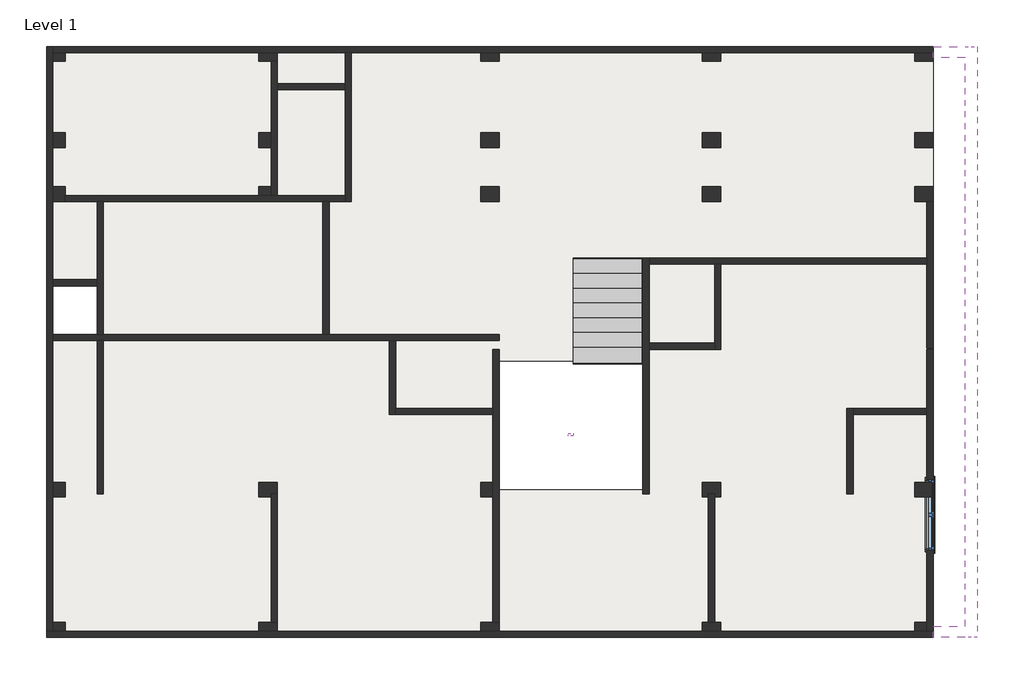
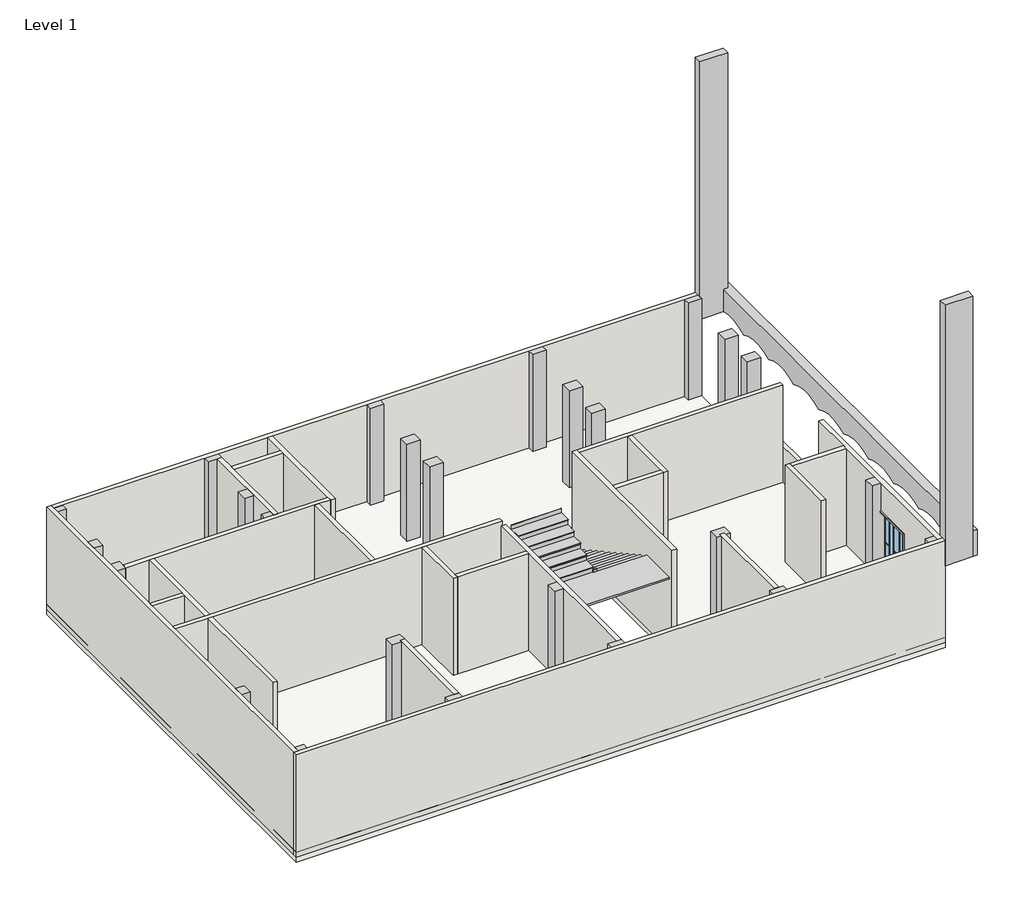
# One storey: 25 columns, 24 walls, 4 proxies, 1 cable carrier fitting, 1 member, 1 slab, 1 stair flight, 1 window.
"""IFC4 building model written with IfcOpenShell, lengths in millimetres."""

from ifc_helpers import new_model, si_unit, frame, origin, origin_with_axes, place, context, project, spatial, polyline, outline, extrude, faceted_brep, transform, mapped, element, save
from components import muntin_pattern_2x2_muntin_pattern_2x2_bff912c5, muntin_pattern_2x2_muntin_pattern_2x2_c2194282, trim_window_exterior_flat_with_sill_e04b3088, trim_window_interior_flat_picture_frame_2a7685fe, conduit_fittings_1_conduit_fittings_1_9411e536, column_family_column_family_eebd7f06, stair_flight_7ee4923a, window_51a0d18f

model = new_model("IFC4")

# Units and contexts
model_context = context("Model", 3, world=origin())
ifc_project = project(units=[si_unit("LENGTHUNIT", "METRE", prefix="MILLI")], contexts=[model_context])

# Site, building, storey
site = spatial("IfcSite", under=ifc_project)
building = spatial("IfcBuilding", under=site)
storey = spatial("IfcBuildingStorey", under=building, Name="Level 1", Elevation=0.0)

# Proxies
placement = place(None, origin())
muntin_pattern_2x2_muntin_pattern_2x2_shape = muntin_pattern_2x2_muntin_pattern_2x2_bff912c5(model_context)
element("IfcBuildingElementProxy", 1, Name="Muntin Pattern_2x2 : Muntin Pattern_2x2", ObjectType="Muntin Pattern_2x2 : Muntin Pattern_2x2", at=placement, inside=storey, context=model_context, shape_type="MappedRepresentation", body=[
    mapped(muntin_pattern_2x2_muntin_pattern_2x2_shape, transform((5833.4324466, -6073.1206508, 417.9089664), x_axis=(0.0, -1.0, 0.0), y_axis=(1.0, 0.0, 0.0), z_axis=(0.0, 0.0, 1.0))),
])
muntin_pattern_2x2_muntin_pattern_2x2_2_shape = muntin_pattern_2x2_muntin_pattern_2x2_c2194282(model_context)
element("IfcBuildingElementProxy", 2, Name="Muntin Pattern_2x2 : Muntin Pattern_2x2", ObjectType="Muntin Pattern_2x2 : Muntin Pattern_2x2", at=placement, inside=storey, context=model_context, shape_type="MappedRepresentation", body=[
    mapped(muntin_pattern_2x2_muntin_pattern_2x2_2_shape, transform((5833.4324466, -6793.8456508, 417.9089664), x_axis=(0.0, 1.0, 0.0), y_axis=(-1.0, 0.0, 0.0), z_axis=(0.0, 0.0, 1.0))),
])
trim_window_exterior_flat_with_sill_shape = trim_window_exterior_flat_with_sill_e04b3088(model_context)
element("IfcBuildingElementProxy", 3, Name="Trim-Window-Exterior-Flat : with Sill", ObjectType="Trim-Window-Exterior-Flat : with Sill", at=placement, inside=storey, context=model_context, shape_type="MappedRepresentation", body=[
    mapped(trim_window_exterior_flat_with_sill_shape, transform((5842.9574466, -6433.4831508, 2176.8589664), x_axis=(0.0, 1.0, 0.0), y_axis=(0.0, 0.0, 1.0), z_axis=(1.0, 0.0, 0.0))),
])
trim_window_interior_flat_picture_frame_shape = trim_window_interior_flat_picture_frame_2a7685fe(model_context)
element("IfcBuildingElementProxy", 4, Name="Trim-Window-Interior-Flat : Picture Frame", ObjectType="Trim-Window-Interior-Flat : Picture Frame", at=placement, inside=storey, context=model_context, shape_type="MappedRepresentation", body=[
    mapped(trim_window_interior_flat_picture_frame_shape, transform((5715.9574466, -6433.4831508, 2176.8589664), x_axis=(0.0, -1.0, 0.0), y_axis=(0.0, 0.0, 1.0), z_axis=(-1.0, 0.0, 0.0))),
])

# Cable carrier fitting
conduit_fittings_1_conduit_fittings_1_shape = conduit_fittings_1_conduit_fittings_1_9411e536(model_context)
element("IfcCableCarrierFitting", 5, ObjectType="Conduit Fittings 1 : Conduit Fittings 1", at=placement, inside=storey, context=model_context, shape_type="MappedRepresentation", body=[
    mapped(conduit_fittings_1_conduit_fittings_1_shape, transform((0.0, 0.0, 0.0), x_axis=(1.0, 0.0, 0.0), y_axis=(0.0, 1.0, 0.0), z_axis=(0.0, 0.0, 1.0))),
])

# Columns
element("IfcColumn", 6, ObjectType="column family : column family", at=placement, inside=storey, context=model_context, shape_type="SweptSolid", body=[
    extrude(outline(polyline([(-12064.0425534, 2926.4168492), (-12318.0425534, 2926.4168492), (-12318.0425534, 3104.2168492), (-12064.0425534, 3104.2168492), (-12064.0425534, 2926.4168492)])), frame((0.0, 0.0, 5.0), z_axis=(0.0, 0.0, 1.0), x_axis=(1.0, 0.0, 0.0)), (0.0, 0.0, 1.0), 3038.0),
])
element("IfcColumn", 7, ObjectType="column family : column family", at=placement, inside=storey, context=model_context, shape_type="SweptSolid", body=[
    extrude(outline(polyline([(-7682.5425534, 2926.4168492), (-8063.5425534, 2926.4168492), (-8063.5425534, 3104.2168492), (-7682.5425534, 3104.2168492), (-7682.5425534, 2926.4168492)])), frame((0.0, 0.0, 5.0), z_axis=(0.0, 0.0, 1.0), x_axis=(1.0, 0.0, 0.0)), (0.0, 0.0, 1.0), 3038.0),
])
element("IfcColumn", 8, ObjectType="column family : column family", at=placement, inside=storey, context=model_context, shape_type="SweptSolid", body=[
    extrude(outline(polyline([(-3110.5425534, 2926.4168492), (-3491.5425534, 2926.4168492), (-3491.5425534, 3104.2168492), (-3110.5425534, 3104.2168492), (-3110.5425534, 2926.4168492)])), frame((0.0, 0.0, 5.0), z_axis=(0.0, 0.0, 1.0), x_axis=(1.0, 0.0, 0.0)), (0.0, 0.0, 1.0), 3038.0),
])
element("IfcColumn", 9, ObjectType="column family : column family", at=placement, inside=storey, context=model_context, shape_type="SweptSolid", body=[
    extrude(outline(polyline([(1461.4574466, 2926.4168492), (1080.4574466, 2926.4168492), (1080.4574466, 3104.2168492), (1461.4574466, 3104.2168492), (1461.4574466, 2926.4168492)])), frame((0.0, 0.0, 5.0), z_axis=(0.0, 0.0, 1.0), x_axis=(1.0, 0.0, 0.0)), (0.0, 0.0, 1.0), 3038.0),
])
element("IfcColumn", 10, ObjectType="column family : column family", at=placement, inside=storey, context=model_context, shape_type="SweptSolid", body=[
    extrude(outline(polyline([(5842.9574466, 2926.4168492), (5461.9574466, 2926.4168492), (5461.9574466, 3104.2168492), (5842.9574466, 3104.2168492), (5842.9574466, 2926.4168492)])), frame((0.0, 0.0, 5.0), z_axis=(0.0, 0.0, 1.0), x_axis=(1.0, 0.0, 0.0)), (0.0, 0.0, 1.0), 3038.0),
])
element("IfcColumn", 11, ObjectType="column family : column family", at=placement, inside=storey, context=model_context, shape_type="SweptSolid", body=[
    extrude(outline(polyline([(-12064.0425534, 335.6168492), (-12064.0425534, 30.8168492), (-12318.0425534, 30.8168492), (-12318.0425534, 335.6168492), (-12064.0425534, 335.6168492)])), frame((0.0, 0.0, 5.0), z_axis=(0.0, 0.0, 1.0), x_axis=(1.0, 0.0, 0.0)), (0.0, 0.0, 1.0), 3038.0),
])
element("IfcColumn", 12, ObjectType="column family : column family", at=placement, inside=storey, context=model_context, shape_type="SweptSolid", body=[
    extrude(outline(polyline([(-12064.0425534, 1449.6754758), (-12064.0425534, 1144.8754758), (-12318.0425534, 1144.8754758), (-12318.0425534, 1449.6754758), (-12064.0425534, 1449.6754758)])), frame((0.0, 0.0, 5.0), z_axis=(0.0, 0.0, 1.0), x_axis=(1.0, 0.0, 0.0)), (0.0, 0.0, 1.0), 3038.0),
])
element("IfcColumn", 13, ObjectType="column family : column family", at=placement, inside=storey, context=model_context, shape_type="SweptSolid", body=[
    extrude(outline(polyline([(-12064.0425534, -5760.3831508), (-12064.0425534, -6065.1831508), (-12318.0425534, -6065.1831508), (-12318.0425534, -5760.3831508), (-12064.0425534, -5760.3831508)])), frame((0.0, 0.0, 5.0), z_axis=(0.0, 0.0, 1.0), x_axis=(1.0, 0.0, 0.0)), (0.0, 0.0, 1.0), 3038.0),
])
element("IfcColumn", 14, ObjectType="column family : column family", at=placement, inside=storey, context=model_context, shape_type="SweptSolid", body=[
    extrude(outline(polyline([(-12064.0425534, -8655.9831508), (-12064.0425534, -8833.7831508), (-12318.0425534, -8833.7831508), (-12318.0425534, -8655.9831508), (-12064.0425534, -8655.9831508)])), frame((0.0, 0.0, 5.0), z_axis=(0.0, 0.0, 1.0), x_axis=(1.0, 0.0, 0.0)), (0.0, 0.0, 1.0), 3038.0),
])
element("IfcColumn", 15, ObjectType="column family : column family", at=placement, inside=storey, context=model_context, shape_type="Brep", body=[
    faceted_brep([(5842.9574466, 335.6168492, 5.0), (5842.9574466, 30.8168492, 5.0), (5461.9574466, 30.8168492, 5.0), (5461.9574466, 335.6168492, 5.0), (5842.9574466, 335.6168492, 3043.0), (5842.9574466, 30.8168492, 3043.0), (5842.9574466, 30.8168492, 1219.2), (5842.9574466, 30.8168492, 152.4), (5461.9574466, 30.8168492, 3043.0), (5461.9574466, 335.6168492, 3043.0)], [[[0, 1, 2, 3]], [[4, 5, 6, 7, 1, 0]], [[5, 8, 2, 1, 7, 6]], [[8, 9, 3, 2]], [[9, 4, 0, 3]], [[4, 9, 8, 5]]]),
])
element("IfcColumn", 16, ObjectType="column family : column family", at=placement, inside=storey, context=model_context, shape_type="SweptSolid", body=[
    extrude(outline(polyline([(5842.9574466, 1449.6754758), (5842.9574466, 1144.8754758), (5461.9574466, 1144.8754758), (5461.9574466, 1449.6754758), (5842.9574466, 1449.6754758)])), frame((0.0, 0.0, 5.0), z_axis=(0.0, 0.0, 1.0), x_axis=(1.0, 0.0, 0.0)), (0.0, 0.0, 1.0), 3038.0),
])
element("IfcColumn", 17, ObjectType="column family : column family", at=placement, inside=storey, context=model_context, shape_type="SweptSolid", body=[
    extrude(outline(polyline([(3043.0, 5461.9574466), (5.0, 5461.9574466), (5.0, 5715.9574466), (348.0589664, 5715.9574466), (348.0589664, 5842.9574466), (2176.8589664, 5842.9574466), (2176.8589664, 5715.9574466), (3043.0, 5715.9574466), (3043.0, 5461.9574466)])), frame((0.0, -6065.1831508, 0.0), z_axis=(0.0, 1.0, 0.0), x_axis=(0.0, 0.0, 1.0)), (0.0, 0.0, 1.0), 304.8),
])
element("IfcColumn", 18, ObjectType="column family : column family", at=placement, inside=storey, context=model_context, shape_type="SweptSolid", body=[
    extrude(outline(polyline([(5461.9574466, -8833.7831508), (5461.9574466, -8655.9831508), (5715.9574466, -8655.9831508), (5715.9574466, -8833.7831508), (5461.9574466, -8833.7831508)])), frame((0.0, 0.0, 5.0), z_axis=(0.0, 0.0, 1.0), x_axis=(1.0, 0.0, 0.0)), (0.0, 0.0, 1.0), 3038.0),
])
element("IfcColumn", 19, ObjectType="column family : column family", at=placement, inside=storey, context=model_context, shape_type="SweptSolid", body=[
    extrude(outline(polyline([(-8063.5425534, -8655.9831508), (-7682.5425534, -8655.9831508), (-7682.5425534, -8833.7831508), (-8063.5425534, -8833.7831508), (-8063.5425534, -8655.9831508)])), frame((0.0, 0.0, 5.0), z_axis=(0.0, 0.0, 1.0), x_axis=(1.0, 0.0, 0.0)), (0.0, 0.0, 1.0), 3038.0),
])
element("IfcColumn", 20, ObjectType="column family : column family", at=placement, inside=storey, context=model_context, shape_type="SweptSolid", body=[
    extrude(outline(polyline([(-3491.5425534, -8655.9831508), (-3110.5425534, -8655.9831508), (-3110.5425534, -8833.7831508), (-3491.5425534, -8833.7831508), (-3491.5425534, -8655.9831508)])), frame((0.0, 0.0, 5.0), z_axis=(0.0, 0.0, 1.0), x_axis=(1.0, 0.0, 0.0)), (0.0, 0.0, 1.0), 3038.0),
])
element("IfcColumn", 21, ObjectType="column family : column family", at=placement, inside=storey, context=model_context, shape_type="SweptSolid", body=[
    extrude(outline(polyline([(1080.4574466, -8655.9831508), (1461.4574466, -8655.9831508), (1461.4574466, -8833.7831508), (1080.4574466, -8833.7831508), (1080.4574466, -8655.9831508)])), frame((0.0, 0.0, 5.0), z_axis=(0.0, 0.0, 1.0), x_axis=(1.0, 0.0, 0.0)), (0.0, 0.0, 1.0), 3038.0),
])
element("IfcColumn", 22, ObjectType="column family : column family", at=placement, inside=storey, context=model_context, shape_type="SweptSolid", body=[
    extrude(outline(polyline([(-8063.5425534, 335.6168492), (-7809.5425534, 335.6168492), (-7809.5425534, 157.8168492), (-8063.5425534, 157.8168492), (-8063.5425534, 335.6168492)])), frame((0.0, 0.0, 5.0), z_axis=(0.0, 0.0, 1.0), x_axis=(1.0, 0.0, 0.0)), (0.0, 0.0, 1.0), 3038.0),
])
element("IfcColumn", 23, ObjectType="column family : column family", at=placement, inside=storey, context=model_context, shape_type="SweptSolid", body=[
    extrude(outline(polyline([(1461.4574466, 335.6168492), (1461.4574466, 30.8168492), (1080.4574466, 30.8168492), (1080.4574466, 335.6168492), (1461.4574466, 335.6168492)])), frame((0.0, 0.0, 5.0), z_axis=(0.0, 0.0, 1.0), x_axis=(1.0, 0.0, 0.0)), (0.0, 0.0, 1.0), 3038.0),
])
element("IfcColumn", 24, ObjectType="column family : column family", at=placement, inside=storey, context=model_context, shape_type="SweptSolid", body=[
    extrude(outline(polyline([(1461.4574466, 1449.6754758), (1461.4574466, 1144.8754758), (1080.4574466, 1144.8754758), (1080.4574466, 1449.6754758), (1461.4574466, 1449.6754758)])), frame((0.0, 0.0, 5.0), z_axis=(0.0, 0.0, 1.0), x_axis=(1.0, 0.0, 0.0)), (0.0, 0.0, 1.0), 3038.0),
])
element("IfcColumn", 25, ObjectType="column family : column family", at=placement, inside=storey, context=model_context, shape_type="SweptSolid", body=[
    extrude(outline(polyline([(-3110.5425534, 1449.6754758), (-3110.5425534, 1144.8754758), (-3491.5425534, 1144.8754758), (-3491.5425534, 1449.6754758), (-3110.5425534, 1449.6754758)])), frame((0.0, 0.0, 5.0), z_axis=(0.0, 0.0, 1.0), x_axis=(1.0, 0.0, 0.0)), (0.0, 0.0, 1.0), 3038.0),
])
element("IfcColumn", 26, ObjectType="column family : column family", at=placement, inside=storey, context=model_context, shape_type="SweptSolid", body=[
    extrude(outline(polyline([(-8063.5425534, 1144.8754758), (-8063.5425534, 1449.6754758), (-7809.5425534, 1449.6754758), (-7809.5425534, 1144.8754758), (-8063.5425534, 1144.8754758)])), frame((0.0, 0.0, 5.0), z_axis=(0.0, 0.0, 1.0), x_axis=(1.0, 0.0, 0.0)), (0.0, 0.0, 1.0), 3038.0),
])
element("IfcColumn", 27, ObjectType="column family : column family", at=placement, inside=storey, context=model_context, shape_type="SweptSolid", body=[
    extrude(outline(polyline([(-8063.5425534, -6065.1831508), (-8063.5425534, -5760.3831508), (-7682.5425534, -5760.3831508), (-7682.5425534, -6001.6831508), (-7809.5425534, -6001.6831508), (-7809.5425534, -6065.1831508), (-8063.5425534, -6065.1831508)])), frame((0.0, 0.0, 5.0), z_axis=(0.0, 0.0, 1.0), x_axis=(1.0, 0.0, 0.0)), (0.0, 0.0, 1.0), 3038.0),
])
element("IfcColumn", 28, ObjectType="column family : column family", at=placement, inside=storey, context=model_context, shape_type="SweptSolid", body=[
    extrude(outline(polyline([(-3491.5425534, -6065.1831508), (-3491.5425534, -5760.3831508), (-3237.5425534, -5760.3831508), (-3237.5425534, -6065.1831508), (-3491.5425534, -6065.1831508)])), frame((0.0, 0.0, 5.0), z_axis=(0.0, 0.0, 1.0), x_axis=(1.0, 0.0, 0.0)), (0.0, 0.0, 1.0), 3038.0),
])
element("IfcColumn", 29, ObjectType="column family : column family", at=placement, inside=storey, context=model_context, shape_type="SweptSolid", body=[
    extrude(outline(polyline([(1461.4574466, -5760.3831508), (1461.4574466, -6065.1831508), (1334.4574466, -6065.1831508), (1334.4574466, -6001.6831508), (1207.4574466, -6001.6831508), (1207.4574466, -6065.1831508), (1080.4574466, -6065.1831508), (1080.4574466, -5760.3831508), (1461.4574466, -5760.3831508)])), frame((0.0, 0.0, 5.0), z_axis=(0.0, 0.0, 1.0), x_axis=(1.0, 0.0, 0.0)), (0.0, 0.0, 1.0), 3038.0),
])
column_family_column_family_shape = column_family_column_family_eebd7f06(model_context)
element("IfcColumn", 30, ObjectType="column family : column family", at=placement, inside=storey, context=model_context, shape_type="MappedRepresentation", body=[
    mapped(column_family_column_family_shape, transform((-3356.6704001, 183.2168492, 0.0), x_axis=(1.0, 0.0, 0.0), y_axis=(0.0, 1.0, 0.0), z_axis=(0.0, 0.0, 1.0))),
])

# Member
element("IfcMember", 31, ObjectType="Stringer - 2\" Width", at=placement, inside=storey, context=model_context, shape_type="SweptSolid", body=[
    extrude(outline(polyline([(-1578.560394, -4757.0831508), (-1578.560394, -4807.8831508), (-1680.160394, -4807.8831508), (-1680.160394, -4757.0831508), (-1578.560394, -4757.0831508)])), frame((0.0, 0.0, 1972.7333333), z_axis=(0.0, 0.0, 1.0), x_axis=(1.0, 0.0, 0.0)), (0.0, 0.0, 1.0), 304.8),
])

# Slab
element("IfcSlab", 32, ObjectType="Generic - 12\" - Filled", at=placement, inside=storey, context=model_context, shape_type="SweptSolid", body=[
    extrude(outline(polyline([(5842.9574466, -8960.7831508), (-12445.0425534, -8960.7831508), (-12445.0425534, 3231.2168492), (5842.9574466, 3231.2168492), (5842.9574466, -8960.7831508)]), holes=[polyline([(-3096.210394, -5912.7831508), (-144.730394, -5912.7831508), (-144.730394, -1135.0431508), (-1578.560394, -1135.0431508), (-1578.560394, -3273.1068434), (-3096.210394, -3273.1068434), (-3096.210394, -5912.7831508)]), polyline([(-11403.6425534, -1709.0831508), (-12318.0425534, -1709.0831508), (-12318.0425534, -2712.3831508), (-11403.6425534, -2712.3831508), (-11403.6425534, -1709.0831508)])]), frame((0.0, 0.0, -152.4), z_axis=(0.0, 0.0, 1.0), x_axis=(1.0, 0.0, 0.0)), (0.0, 0.0, 1.0), 304.8),
])

# Stair flight
stair_flight_shape = stair_flight_7ee4923a(model_context)
element("IfcStairFlight", 33, ObjectType="2\" Tread 1\" Nosing 1/4\" Riser", at=placement, inside=storey, context=model_context, shape_type="MappedRepresentation", body=[
    mapped(stair_flight_shape, transform((0.0, 0.0, 0.0), x_axis=(1.0, 0.0, 0.0), y_axis=(0.0, 1.0, 0.0), z_axis=(0.0, 0.0, 1.0))),
])

# Walls
element("IfcWall", 34, ObjectType="Generic - 5\"", at=placement, inside=storey, context=model_context, shape_type="Brep", body=[
    faceted_brep([(-12445.0425534, -8960.7831508, 0.0), (5842.9574466, -8960.7831508, 0.0), (5842.9574466, -8960.7831508, 3048.0), (-12445.0425534, -8960.7831508, 3048.0), (-12445.0425534, -8833.7831508, 0.0), (-12445.0425534, -8833.7831508, 3048.0), (-12318.0425534, -8833.7831508, 3048.0), (5715.9574466, -8833.7831508, 3048.0), (5842.9574466, -8833.7831508, 3048.0), (5842.9574466, -8833.7831508, 0.0), (5715.9574466, -8833.7831508, 0.0), (-12318.0425534, -8833.7831508, 0.0)], [[[0, 1, 2, 3]], [[4, 5, 6, 7, 8, 9, 10, 11]], [[1, 0, 4, 11, 10, 9]], [[3, 2, 8, 7, 6, 5]], [[2, 1, 9, 8]], [[0, 3, 5, 4]]]),
])
element("IfcWall", 35, ObjectType="Generic - 5\"", at=placement, inside=storey, context=model_context, shape_type="Brep", body=[
    faceted_brep([(5842.9574466, -8833.7831508, 0.0), (5842.9574466, -3017.1831508, 0.0), (5842.9574466, -3017.1831508, 3048.0), (5842.9574466, -8833.7831508, 3048.0), (5842.9574466, -7157.3831508, 2176.8589664), (5842.9574466, -6065.1831508, 2176.8589664), (5842.9574466, -5760.3831508, 2176.8589664), (5842.9574466, -5709.5831508, 2176.8589664), (5842.9574466, -5709.5831508, 348.0589664), (5842.9574466, -5760.3831508, 348.0589664), (5842.9574466, -6065.1831508, 348.0589664), (5842.9574466, -7157.3831508, 348.0589664), (5715.9574466, -8833.7831508, 0.0), (5715.9574466, -8833.7831508, 5.0), (5715.9574466, -8833.7831508, 3043.0), (5715.9574466, -8833.7831508, 3048.0), (5715.9574466, -4363.3831508, 3048.0), (5715.9574466, -4236.3831508, 3048.0), (5715.9574466, -3017.1831508, 3048.0), (5715.9574466, -3017.1831508, 0.0), (5715.9574466, -4236.3831508, 0.0), (5715.9574466, -4363.3831508, 0.0), (5715.9574466, -7157.3831508, 2176.8589664), (5715.9574466, -7157.3831508, 348.0589664), (5715.9574466, -6065.1831508, 348.0589664), (5715.9574466, -5760.3831508, 348.0589664), (5715.9574466, -5709.5831508, 348.0589664), (5715.9574466, -5709.5831508, 2176.8589664), (5715.9574466, -5760.3831508, 2176.8589664), (5715.9574466, -6065.1831508, 2176.8589664)], [[[0, 1, 2, 3], [4, 5, 6, 7, 8, 9, 10, 11]], [[12, 13, 14, 15, 16, 17, 18, 19, 20, 21], [22, 23, 24, 25, 26, 27, 28, 29]], [[1, 0, 12, 21, 20, 19]], [[2, 1, 19, 18]], [[3, 2, 18, 17, 16, 15]], [[0, 3, 15, 14, 13, 12]], [[23, 22, 4, 11]], [[26, 25, 24, 23, 11, 10, 9, 8]], [[27, 26, 8, 7]], [[22, 29, 28, 27, 7, 6, 5, 4]]]),
])
element("IfcWall", 36, ObjectType="Generic - 5\"", at=placement, inside=storey, context=model_context, shape_type="Brep", body=[
    faceted_brep([(-12318.0425534, -8833.7831508, 0.0), (-12318.0425534, -2839.3831508, 0.0), (-12318.0425534, -2712.3831508, 0.0), (-12318.0425534, -1709.0831508, 0.0), (-12318.0425534, -1582.0831508, 0.0), (-12318.0425534, 3104.2168492, 0.0), (-12318.0425534, 3231.2168492, 0.0), (-12318.0425534, 3231.2168492, 3048.0), (-12318.0425534, 3104.2168492, 3048.0), (-12318.0425534, -1582.0831508, 3048.0), (-12318.0425534, -1709.0831508, 3048.0), (-12318.0425534, -2712.3831508, 3048.0), (-12318.0425534, -2839.3831508, 3048.0), (-12318.0425534, -8833.7831508, 3048.0), (-12318.0425534, -8833.7831508, 3043.0), (-12318.0425534, -8833.7831508, 5.0), (-12445.0425534, -8833.7831508, 0.0), (-12445.0425534, -8833.7831508, 3048.0), (-12445.0425534, 3231.2168492, 3048.0), (-12445.0425534, 3231.2168492, 0.0)], [[[0, 1, 2, 3, 4, 5, 6, 7, 8, 9, 10, 11, 12, 13, 14, 15]], [[16, 17, 18, 19]], [[6, 5, 4, 3, 2, 1, 0, 16, 19]], [[13, 12, 11, 10, 9, 8, 7, 18, 17]], [[0, 15, 14, 13, 17, 16]], [[7, 6, 19, 18]]]),
])
element("IfcWall", 37, ObjectType="Generic - 5\"", at=placement, inside=storey, context=model_context, shape_type="Brep", body=[
    faceted_brep([(-12318.0425534, 3104.2168492, 0.0), (-6285.5425534, 3104.2168492, 0.0), (-6158.5425534, 3104.2168492, 0.0), (5842.9574466, 3104.2168492, 0.0), (5842.9574466, 3104.2168492, 5.0), (5842.9574466, 3104.2168492, 3043.0), (5842.9574466, 3104.2168492, 3048.0), (-6158.5425534, 3104.2168492, 3048.0), (-6285.5425534, 3104.2168492, 3048.0), (-12318.0425534, 3104.2168492, 3048.0), (-12318.0425534, 3104.2168492, 3043.0), (-12318.0425534, 3104.2168492, 5.0), (-12318.0425534, 3231.2168492, 0.0), (-12318.0425534, 3231.2168492, 3048.0), (5842.9574466, 3231.2168492, 3048.0), (5842.9574466, 3231.2168492, 0.0)], [[[0, 1, 2, 3, 4, 5, 6, 7, 8, 9, 10, 11]], [[12, 13, 14, 15]], [[3, 2, 1, 0, 12, 15]], [[6, 5, 4, 3, 15, 14]], [[9, 8, 7, 6, 14, 13]], [[0, 11, 10, 9, 13, 12]]]),
])
element("IfcWall", 38, ObjectType="Generic - 5\"", at=placement, inside=storey, context=model_context, shape_type="SweptSolid", body=[
    extrude(outline(polyline([(5842.9574466, 30.8168492), (5842.9574466, -2991.7831508), (5715.9574466, -2991.7831508), (5715.9574466, 30.8168492), (5842.9574466, 30.8168492)])), frame((0.0, 0.0, 152.4), z_axis=(0.0, 0.0, 1.0), x_axis=(1.0, 0.0, 0.0)), (0.0, 0.0, 1.0), 1066.8),
])
element("IfcWall", 39, ObjectType="Generic - 5\"", at=placement, inside=storey, context=model_context, shape_type="Brep", body=[
    faceted_brep([(-3110.5425534, -2712.3831508, 0.0), (-6615.7425534, -2712.3831508, 0.0), (-6742.7425534, -2712.3831508, 0.0), (-11276.6425534, -2712.3831508, 0.0), (-11403.6425534, -2712.3831508, 0.0), (-12318.0425534, -2712.3831508, 0.0), (-12318.0425534, -2712.3831508, 3048.0), (-11403.6425534, -2712.3831508, 3048.0), (-11276.6425534, -2712.3831508, 3048.0), (-6742.7425534, -2712.3831508, 3048.0), (-6615.7425534, -2712.3831508, 3048.0), (-3110.5425534, -2712.3831508, 3048.0), (-3110.5425534, -2839.3831508, 0.0), (-3110.5425534, -2839.3831508, 3048.0), (-5244.1425534, -2839.3831508, 3048.0), (-5371.1425534, -2839.3831508, 3048.0), (-11276.6425534, -2839.3831508, 3048.0), (-11403.6425534, -2839.3831508, 3048.0), (-12318.0425534, -2839.3831508, 3048.0), (-12318.0425534, -2839.3831508, 0.0), (-11403.6425534, -2839.3831508, 0.0), (-11276.6425534, -2839.3831508, 0.0), (-5371.1425534, -2839.3831508, 0.0), (-5244.1425534, -2839.3831508, 0.0)], [[[0, 1, 2, 3, 4, 5, 6, 7, 8, 9, 10, 11]], [[12, 13, 14, 15, 16, 17, 18, 19, 20, 21, 22, 23]], [[5, 4, 3, 2, 1, 0, 12, 23, 22, 21, 20, 19]], [[11, 10, 9, 8, 7, 6, 18, 17, 16, 15, 14, 13]], [[0, 11, 13, 12]], [[6, 5, 19, 18]]]),
])
element("IfcWall", 40, ObjectType="Generic - 5\"", at=placement, inside=storey, context=model_context, shape_type="Brep", body=[
    faceted_brep([(-5371.1425534, -2839.3831508, 0.0), (-5371.1425534, -4363.3831508, 0.0), (-5371.1425534, -4363.3831508, 3048.0), (-5371.1425534, -2839.3831508, 3048.0), (-5244.1425534, -2839.3831508, 0.0), (-5244.1425534, -2839.3831508, 3048.0), (-5244.1425534, -4236.3831508, 3048.0), (-5244.1425534, -4363.3831508, 3048.0), (-5244.1425534, -4363.3831508, 0.0), (-5244.1425534, -4236.3831508, 0.0)], [[[0, 1, 2, 3]], [[4, 5, 6, 7, 8, 9]], [[1, 0, 4, 9, 8]], [[3, 2, 7, 6, 5]], [[0, 3, 5, 4]], [[2, 1, 8, 7]]]),
])
element("IfcWall", 41, ObjectType="Generic - 5\"", at=placement, inside=storey, context=model_context, shape_type="Brep", body=[
    faceted_brep([(-7809.5425534, 2926.4168492, 0.0), (-7809.5425534, 157.8168492, 0.0), (-7809.5425534, 157.8168492, 5.0), (-7809.5425534, 157.8168492, 3043.0), (-7809.5425534, 157.8168492, 3048.0), (-7809.5425534, 2926.4168492, 3048.0), (-7682.5425534, 2926.4168492, 0.0), (-7682.5425534, 2926.4168492, 5.0), (-7682.5425534, 2926.4168492, 3043.0), (-7682.5425534, 2926.4168492, 3048.0), (-7682.5425534, 2469.2168492, 3048.0), (-7682.5425534, 2342.2168492, 3048.0), (-7682.5425534, 157.8168492, 3048.0), (-7682.5425534, 157.8168492, 0.0), (-7682.5425534, 2342.2168492, 0.0), (-7682.5425534, 2469.2168492, 0.0)], [[[0, 1, 2, 3, 4, 5]], [[6, 7, 8, 9, 10, 11, 12, 13, 14, 15]], [[1, 0, 6, 15, 14, 13]], [[5, 4, 12, 11, 10, 9]], [[0, 5, 9, 8, 7, 6]], [[4, 3, 2, 1, 13, 12]]]),
])
element("IfcWall", 42, ObjectType="Generic - 5\"", at=placement, inside=storey, context=model_context, shape_type="Brep", body=[
    faceted_brep([(-12064.0425534, 30.8168492, 0.0), (-11403.6425534, 30.8168492, 0.0), (-11276.6425534, 30.8168492, 0.0), (-6742.7425534, 30.8168492, 0.0), (-6615.7425534, 30.8168492, 0.0), (-6285.5425534, 30.8168492, 0.0), (-6285.5425534, 30.8168492, 3048.0), (-6615.7425534, 30.8168492, 3048.0), (-6742.7425534, 30.8168492, 3048.0), (-11276.6425534, 30.8168492, 3048.0), (-11403.6425534, 30.8168492, 3048.0), (-12064.0425534, 30.8168492, 3048.0), (-12064.0425534, 30.8168492, 3043.0), (-12064.0425534, 30.8168492, 5.0), (-12064.0425534, 157.8168492, 0.0), (-12064.0425534, 157.8168492, 3048.0), (-7809.5425534, 157.8168492, 3048.0), (-7682.5425534, 157.8168492, 3048.0), (-6285.5425534, 157.8168492, 3048.0), (-6285.5425534, 157.8168492, 0.0), (-7682.5425534, 157.8168492, 0.0), (-7809.5425534, 157.8168492, 0.0)], [[[0, 1, 2, 3, 4, 5, 6, 7, 8, 9, 10, 11, 12, 13]], [[14, 15, 16, 17, 18, 19, 20, 21]], [[5, 4, 3, 2, 1, 0, 14, 21, 20, 19]], [[11, 10, 9, 8, 7, 6, 18, 17, 16, 15]], [[0, 13, 12, 11, 15, 14]], [[6, 5, 19, 18]]]),
])
element("IfcWall", 43, ObjectType="Generic - 5\"", at=placement, inside=storey, context=model_context, shape_type="SweptSolid", body=[
    extrude(outline(polyline([(-3237.5425534, -4363.3831508), (-5244.1425534, -4363.3831508), (-5244.1425534, -4236.3831508), (-3237.5425534, -4236.3831508), (-3237.5425534, -4363.3831508)])), origin_with_axes(), (0.0, 0.0, 1.0), 3048.0),
])
element("IfcWall", 44, ObjectType="Generic - 5\"", at=placement, inside=storey, context=model_context, shape_type="Brep", body=[
    faceted_brep([(-3237.5425534, -3017.1831508, 0.0), (-3237.5425534, -4236.3831508, 0.0), (-3237.5425534, -4363.3831508, 0.0), (-3237.5425534, -8655.9831508, 0.0), (-3237.5425534, -8655.9831508, 3048.0), (-3237.5425534, -4363.3831508, 3048.0), (-3237.5425534, -4236.3831508, 3048.0), (-3237.5425534, -3017.1831508, 3048.0), (-3110.5425534, -3017.1831508, 0.0), (-3110.5425534, -3017.1831508, 3048.0), (-3110.5425534, -8655.9831508, 3048.0), (-3110.5425534, -8655.9831508, 3043.0), (-3110.5425534, -8655.9831508, 5.0), (-3110.5425534, -8655.9831508, 0.0)], [[[0, 1, 2, 3, 4, 5, 6, 7]], [[8, 9, 10, 11, 12, 13]], [[3, 2, 1, 0, 8, 13]], [[4, 3, 13, 12, 11, 10]], [[7, 6, 5, 4, 10, 9]], [[0, 7, 9, 8]]]),
])
element("IfcWall", 45, ObjectType="Generic - 5\"", at=placement, inside=storey, context=model_context, shape_type="Brep", body=[
    faceted_brep([(-7809.5425534, -6001.6831508, 0.0), (-7809.5425534, -8655.9831508, 0.0), (-7809.5425534, -8655.9831508, 3048.0), (-7809.5425534, -6001.6831508, 3048.0), (-7809.5425534, -6001.6831508, 3043.0), (-7809.5425534, -6001.6831508, 5.0), (-7682.5425534, -6001.6831508, 0.0), (-7682.5425534, -6001.6831508, 5.0), (-7682.5425534, -6001.6831508, 3043.0), (-7682.5425534, -6001.6831508, 3048.0), (-7682.5425534, -8655.9831508, 3048.0), (-7682.5425534, -8655.9831508, 3043.0), (-7682.5425534, -8655.9831508, 5.0), (-7682.5425534, -8655.9831508, 0.0)], [[[0, 1, 2, 3, 4, 5]], [[6, 7, 8, 9, 10, 11, 12, 13]], [[1, 0, 6, 13]], [[2, 1, 13, 12, 11, 10]], [[3, 2, 10, 9]], [[0, 5, 4, 3, 9, 8, 7, 6]]]),
])
element("IfcWall", 46, ObjectType="Generic - 5\"", at=placement, inside=storey, context=model_context, shape_type="SweptSolid", body=[
    extrude(outline(polyline([(-6742.7425534, -2712.3831508), (-6742.7425534, 30.8168492), (-6615.7425534, 30.8168492), (-6615.7425534, -2712.3831508), (-6742.7425534, -2712.3831508)])), origin_with_axes(), (0.0, 0.0, 1.0), 3048.0),
])
element("IfcWall", 47, ObjectType="Generic - 5\"", at=placement, inside=storey, context=model_context, shape_type="Brep", body=[
    faceted_brep([(-11403.6425534, -6001.6831508, 0.0), (-11403.6425534, -6001.6831508, 3048.0), (-11403.6425534, -2839.3831508, 3048.0), (-11403.6425534, -2839.3831508, 0.0), (-11276.6425534, -6001.6831508, 3048.0), (-11276.6425534, -6001.6831508, 0.0), (-11276.6425534, -2839.3831508, 0.0), (-11276.6425534, -2839.3831508, 3048.0)], [[[0, 1, 2, 3]], [[4, 5, 6, 7]], [[5, 0, 3, 6]], [[1, 0, 5, 4]], [[1, 4, 7, 2]], [[3, 2, 7, 6]]]),
    faceted_brep([(-11403.6425534, 30.8168492, 3048.0), (-11403.6425534, 30.8168492, 0.0), (-11403.6425534, -1582.0831508, 0.0), (-11403.6425534, -1709.0831508, 0.0), (-11403.6425534, -2712.3831508, 0.0), (-11403.6425534, -2712.3831508, 3048.0), (-11403.6425534, -1709.0831508, 3048.0), (-11403.6425534, -1582.0831508, 3048.0), (-11276.6425534, 30.8168492, 0.0), (-11276.6425534, 30.8168492, 3048.0), (-11276.6425534, -2712.3831508, 3048.0), (-11276.6425534, -2712.3831508, 0.0)], [[[0, 1, 2, 3, 4, 5, 6, 7]], [[8, 9, 10, 11]], [[1, 8, 11, 4, 3, 2]], [[9, 0, 7, 6, 5, 10]], [[1, 0, 9, 8]], [[5, 4, 11, 10]]]),
])
element("IfcWall", 48, ObjectType="Generic - 5\"", at=placement, inside=storey, context=model_context, shape_type="SweptSolid", body=[
    extrude(outline(polyline([(-12318.0425534, -1582.0831508), (-11403.6425534, -1582.0831508), (-11403.6425534, -1709.0831508), (-12318.0425534, -1709.0831508), (-12318.0425534, -1582.0831508)])), origin_with_axes(), (0.0, 0.0, 1.0), 3048.0),
])
element("IfcWall", 49, ObjectType="Generic - 5\"", at=placement, inside=storey, context=model_context, shape_type="Brep", body=[
    faceted_brep([(-6285.5425534, 3104.2168492, 0.0), (-6285.5425534, 2469.2168492, 0.0), (-6285.5425534, 2342.2168492, 0.0), (-6285.5425534, 157.8168492, 0.0), (-6285.5425534, 30.8168492, 0.0), (-6285.5425534, 30.8168492, 3048.0), (-6285.5425534, 157.8168492, 3048.0), (-6285.5425534, 2342.2168492, 3048.0), (-6285.5425534, 2469.2168492, 3048.0), (-6285.5425534, 3104.2168492, 3048.0), (-6158.5425534, 3104.2168492, 0.0), (-6158.5425534, 3104.2168492, 3048.0), (-6158.5425534, 30.8168492, 3048.0), (-6158.5425534, 30.8168492, 0.0)], [[[0, 1, 2, 3, 4, 5, 6, 7, 8, 9]], [[10, 11, 12, 13]], [[4, 3, 2, 1, 0, 10, 13]], [[9, 8, 7, 6, 5, 12, 11]], [[0, 9, 11, 10]], [[5, 4, 13, 12]]]),
])
element("IfcWall", 50, ObjectType="Generic - 5\"", at=placement, inside=storey, context=model_context, shape_type="SweptSolid", body=[
    extrude(outline(polyline([(-6285.5425534, 2342.2168492), (-7682.5425534, 2342.2168492), (-7682.5425534, 2469.2168492), (-6285.5425534, 2469.2168492), (-6285.5425534, 2342.2168492)])), origin_with_axes(), (0.0, 0.0, 1.0), 3048.0),
])
element("IfcWall", 51, ObjectType="Generic - 5\"", at=placement, inside=storey, context=model_context, shape_type="Brep", body=[
    faceted_brep([(-17.730394, -1262.0431508, 0.0), (1334.4574466, -1262.0431508, 0.0), (1461.4574466, -1262.0431508, 0.0), (5715.9574466, -1262.0431508, 0.0), (5715.9574466, -1262.0431508, 3048.0), (1461.4574466, -1262.0431508, 3048.0), (1334.4574466, -1262.0431508, 3048.0), (-17.730394, -1262.0431508, 3048.0), (-17.730394, -1135.0431508, 0.0), (-17.730394, -1135.0431508, 3048.0), (5715.9574466, -1135.0431508, 3048.0), (5715.9574466, -1135.0431508, 0.0)], [[[0, 1, 2, 3, 4, 5, 6, 7]], [[8, 9, 10, 11]], [[3, 2, 1, 0, 8, 11]], [[7, 6, 5, 4, 10, 9]], [[0, 7, 9, 8]], [[4, 3, 11, 10]]]),
])
element("IfcWall", 52, ObjectType="Generic - 5\"", at=placement, inside=storey, context=model_context, shape_type="Brep", body=[
    faceted_brep([(1207.4574466, -6001.6831508, 0.0), (1207.4574466, -8655.9831508, 0.0), (1207.4574466, -8655.9831508, 3048.0), (1207.4574466, -6001.6831508, 3048.0), (1207.4574466, -6001.6831508, 3043.0), (1207.4574466, -6001.6831508, 5.0), (1334.4574466, -6001.6831508, 0.0), (1334.4574466, -6001.6831508, 5.0), (1334.4574466, -6001.6831508, 3043.0), (1334.4574466, -6001.6831508, 3048.0), (1334.4574466, -8655.9831508, 3048.0), (1334.4574466, -8655.9831508, 0.0)], [[[0, 1, 2, 3, 4, 5]], [[6, 7, 8, 9, 10, 11]], [[1, 0, 6, 11]], [[2, 1, 11, 10]], [[3, 2, 10, 9]], [[0, 5, 4, 3, 9, 8, 7, 6]]]),
])
element("IfcWall", 53, ObjectType="Generic - 5\"", at=placement, inside=storey, context=model_context, shape_type="Brep", body=[
    faceted_brep([(-17.730394, -6001.6831508, 0.0), (-17.730394, -3017.1831508, 0.0), (-17.730394, -2890.1831508, 0.0), (-17.730394, -1262.0431508, 0.0), (-17.730394, -1135.0431508, 0.0), (-17.730394, -1135.0431508, 3048.0), (-17.730394, -1262.0431508, 3048.0), (-17.730394, -2890.1831508, 3048.0), (-17.730394, -3017.1831508, 3048.0), (-17.730394, -6001.6831508, 3048.0), (-144.730394, -6001.6831508, 0.0), (-144.730394, -6001.6831508, 3048.0), (-144.730394, -1135.0431508, 3048.0), (-144.730394, -1135.0431508, 0.0)], [[[0, 1, 2, 3, 4, 5, 6, 7, 8, 9]], [[10, 11, 12, 13]], [[4, 3, 2, 1, 0, 10, 13]], [[9, 8, 7, 6, 5, 12, 11]], [[0, 9, 11, 10]], [[5, 4, 13, 12]]]),
])
element("IfcWall", 54, ObjectType="Generic - 5\"", at=placement, inside=storey, context=model_context, shape_type="Brep", body=[
    faceted_brep([(4064.9574466, -4236.3831508, 0.0), (4064.9574466, -6001.6831508, 0.0), (4064.9574466, -6001.6831508, 3048.0), (4064.9574466, -4236.3831508, 3048.0), (4191.9574466, -4236.3831508, 0.0), (4191.9574466, -4236.3831508, 3048.0), (4191.9574466, -4363.3831508, 3048.0), (4191.9574466, -6001.6831508, 3048.0), (4191.9574466, -6001.6831508, 0.0), (4191.9574466, -4363.3831508, 0.0)], [[[0, 1, 2, 3]], [[4, 5, 6, 7, 8, 9]], [[1, 0, 4, 9, 8]], [[2, 1, 8, 7]], [[3, 2, 7, 6, 5]], [[0, 3, 5, 4]]]),
])
element("IfcWall", 55, ObjectType="Generic - 5\"", at=placement, inside=storey, context=model_context, shape_type="SweptSolid", body=[
    extrude(outline(polyline([(5715.9574466, -4363.3831508), (4191.9574466, -4363.3831508), (4191.9574466, -4236.3831508), (5715.9574466, -4236.3831508), (5715.9574466, -4363.3831508)])), origin_with_axes(), (0.0, 0.0, 1.0), 3048.0),
])
element("IfcWall", 56, ObjectType="Generic - 5\"", at=placement, inside=storey, context=model_context, shape_type="Brep", body=[
    faceted_brep([(1334.4574466, -1262.0431508, 0.0), (1334.4574466, -2890.1831508, 0.0), (1334.4574466, -3017.1831508, 0.0), (1334.4574466, -3017.1831508, 3048.0), (1334.4574466, -2890.1831508, 3048.0), (1334.4574466, -1262.0431508, 3048.0), (1461.4574466, -1262.0431508, 0.0), (1461.4574466, -1262.0431508, 3048.0), (1461.4574466, -3017.1831508, 3048.0), (1461.4574466, -3017.1831508, 0.0)], [[[0, 1, 2, 3, 4, 5]], [[6, 7, 8, 9]], [[2, 1, 0, 6, 9]], [[5, 4, 3, 8, 7]], [[0, 5, 7, 6]], [[3, 2, 9, 8]]]),
])
element("IfcWall", 57, ObjectType="Generic - 5\"", at=placement, inside=storey, context=model_context, shape_type="SweptSolid", body=[
    extrude(outline(polyline([(-17.730394, -2890.1831508), (1334.4574466, -2890.1831508), (1334.4574466, -3017.1831508), (-17.730394, -3017.1831508), (-17.730394, -2890.1831508)])), origin_with_axes(), (0.0, 0.0, 1.0), 3048.0),
])

# Window
window_shape = window_51a0d18f(model_context)
element("IfcWindow", 58, ObjectType="Window-Casement-Double : 57\" x 72\"", at=placement, inside=storey, context=model_context, shape_type="MappedRepresentation", body=[
    mapped(window_shape, transform((5779.4574466, -6433.4831508, -566.3410336), x_axis=(0.0, -1.0, 0.0), y_axis=(1.0, 0.0, 0.0), z_axis=(0.0, 0.0, 1.0))),
])

save(model, "model.ifc")

# Revit data of these elements
# Grids (mm)
#   "2": line (-7873.043, -12499.654) -> (-7873.043, 11064.123)
#   "3": line (-3301.043, -12499.654) -> (-3301.043, 11064.123)
#   "4": line (1270.957, -12499.654) -> (1270.957, 11064.123)
#   "5": line (5842.957, -12499.654) -> (5842.957, 11064.123)
#   "7": line (9725.823, 183.217) -> (-17423.972, 183.217)
#   "10": line (9725.823, -8960.783) -> (-17423.972, -8960.783)
#   "6": line (9725.823, 3231.217) -> (-17423.972, 3231.217)
#   "8": line (11985.226, 1297.275) -> (-15164.569, 1297.275)
#   "9": line (9725.823, -5912.783) -> (-17423.972, -5912.783)
# Type "Muntin Pattern_2x2 : Muntin Pattern_2x2"
#   Width [instance default] = 4' - 0"
#   Thickness = 0' - 0 1/2"
#   Height [instance default] = 4' - 0"
#   Distance = 0' - 0 3/4"
#   Interior Material [instance default] = none
#   Exterior Material [instance default] = none
#   Default Elevation = 0
# Type "Trim-Window-Exterior-Flat : with Sill"
#   Trim Width = 0' - 2 1/4"
#   Trim Thickness_Picture Frame = 0' - 1 1/4"
#   Trim Thickness_with Sill = 0' - 0 3/4"
#   Sill Thickness = 0' - 1 1/4"
#   Opening Width [instance default] = 2' - 0"
#   Opening Height [instance default] = 3' - 0"
#   Default Elevation = 4' - 0"
#   Sill = yes
#   Picture Frame = no
#   Trim Material [instance default] = none
# Type "Trim-Window-Interior-Flat : Picture Frame"
#   Trim Thickness_Picture Frame = 0' - 1 1/4"
#   Trim Width = 0' - 2 1/4"
#   Trim Thickness_with Sill = 0' - 0 3/4"
#   Sill Thickness = 0' - 1 1/4"
#   Opening Width [instance default] = 2' - 0"
#   Opening Height [instance default] = 3' - 0"
#   Default Elevation = 4' - 0"
#   Sill = no
#   Picture Frame = yes
#   Trim Material [instance default] = none
# Type "column family : column family"
#   w2 [instance default] = 0' - 9.88189"
#   w1 [instance default] = 0' - 9.01575"
#   Depth = 1' - 11.62205"
#   Width = 1' - 11.62205"
# Type "Generic - 12\" - Filled"
#   Assembly Code = "B1010"
#   Function = 0
#   Layers, outside or top first: 1' - 0" no material (function 1)
# Type "Generic - 5\""
#   Assembly Code = "B2010"
#   Layers, outside or top first: 0' - 5" no material (function 1)
# Type "Window-Casement-Double : 57\" x 72\""
#   Type Mark = "17"
#   Fire Rating = "0.5h"
#   Assembly Code = "B2020100"
#   Analytic Construction = "Double glazing - domestic"
#   Frame Extension [instance default] = 0' - 0 1/4"
#   Window Inset [instance default] = 0' - 0"
#   Wall Thickness [instance default] = 0' - 6"
#   Interior Wall Closure [instance default] = 0' - 2 1/4"
#   Half Width = 2' - 4 1/2"
#   Visual Light Transmittance = 0.81
#   Thermal Resistance (R) = 1.8146 (h·ft²·°F)/BTU
#   Solar Heat Gain Coefficient = 0.76
#   Rough Width = 4' - 9 1/2"
#   Rough Height = 6' - 0 1/2"
#   Height = 6' - 0"
#   Heat Transfer Coefficient (U) = 0.5511 BTU/(h·ft²·°F)
#   Exterior Wall Closure [instance default] = 0' - 1 1/4"
#   Extension Jamb [instance default] = 0' - 2 1/4"
#   Default Sill Height = 3' - 0"
#   Width = 4' - 9"
#   Define Thermal Properties by = 0
#   Muntin Visibility = yes
#   Interior Trim Visibility [instance default] = yes
#   Exterior Trim Visibility [instance default] = yes
#   Extension Jamb Visibility [instance default] = yes
#   Interior Trim Material = Wood - Stained
#   Muntin Pattern = Muntin Pattern_2x2 : Muntin Pattern_2x2
#   Interior Trim = Trim-Window-Interior-Flat : Picture Frame
#   Interior Frame Material = Wood - Stained
#   Glass Panel Material = Glass
#   Exterior Trim Material = Clad - White
#   Exterior Trim = Trim-Window-Exterior-Flat : with Sill
#   Exterior Frame Material = Clad - White
#   Wall Closure = (empty or 0)
# Elements 1, 2 (IfcBuildingElementProxy, "Muntin Pattern_2x2 : Muntin Pattern_2x2")
#   Width = 1' - 11 1/8"
#   Height = 5' - 6 1/2"
#   Interior Material = Wood - Stained
#   Exterior Material = Clad - White
#   Phase Created = New Construction
#   Materials on its faces: "Clad - White", "Wood - Stained"
# Element 3 (IfcBuildingElementProxy, "Trim-Window-Exterior-Flat : with Sill")
#   Opening Width = 4' - 9"
#   Opening Height = 6' - 0"
#   Trim Material = Clad - White
#   Phase Created = New Construction
#   Materials on its faces: "Clad - White"
# Element 4 (IfcBuildingElementProxy, "Trim-Window-Interior-Flat : Picture Frame")
#   Opening Width = 4' - 9"
#   Opening Height = 6' - 0"
#   Trim Material = Wood - Stained
#   Phase Created = New Construction
#   Materials on its faces: "Wood - Stained"
# Element 5 (IfcCableCarrierFitting, "Conduit Fittings 1 : Conduit Fittings 1")
#   built-in parameter 1140129 = 2
#   Phase Created = New Construction
# Elements 6, 7, 8, 9, 10, 11, 12, 13, 14, 17, 18, 19, 20, 21, 22, 26, 27, 28, 29 (IfcColumn, "column family : column family")
#   w2 = 1' - 0"
#   w1 = 1' - 3"
#   Phase Created = New Construction
#   Materials on its faces: "Default Wall"
# Element 15 (IfcColumn, "column family : column family")
#   w2 = 1' - 0"
#   w1 = 1' - 3"
#   Phase Created = New Construction
#   Materials on its faces: "cream colour", "Default Wall"
# Elements 16, 23, 24, 25, 30 (IfcColumn, "column family : column family")
#   w2 = 1' - 0"
#   w1 = 1' - 3"
#   Phase Created = New Construction
# Element 31 (IfcMember, "Stringer - 2\" Width")
#   Phase Created = New Construction
# Element 32 (IfcSlab, "Generic - 12\" - Filled")
#   Height Offset From Level = 0' - 6"
#   Phase Created = New Construction
#   Materials on its faces: "Default Floor", "Wood - Stained"
# Element 33 (IfcStairFlight, "2\" Tread 1\" Nosing 1/4\" Riser")
#   Phase Created = New Construction
# Elements 34, 36, 37 (IfcWall, "Generic - 5\"")
#   Top Offset = 0' - 0"
#   Base Offset = 0' - 0"
#   wall height = 10' - 0"
#   Phase Created = New Construction
#   Base Constraint = Level 1
#   Top Constraint = Level 2
#   Materials on its faces: "Default Wall", "cream colour"
# Elements 35, 39, 40, 41, 42, 43, 44, 45, 46, 47, 48, 49, 50, 51, 52, 53, 54, 55, 56, 57 (IfcWall, "Generic - 5\"")
#   Top Offset = 0' - 0"
#   Base Offset = 0' - 0"
#   wall height = 10' - 0"
#   Phase Created = New Construction
#   Base Constraint = Level 1
#   Top Constraint = Level 2
#   Materials on its faces: "Default Wall"
# Element 38 (IfcWall, "Generic - 5\"")
#   built-in parameter 1001111 = 0' - 6"
#   Top Offset = 0' - 0"
#   Base Offset = 0' - 6"
#   Unconnected Height = 3' - 6"
#   wall height = 3' - 6"
#   Phase Created = New Construction
#   Base Constraint = Level 1
#   Materials on its faces: "Default Wall", "cream colour"
# Element 58 (IfcWindow, "Window-Casement-Double : 57\" x 72\"")
#   Mark = "22"
#   Window Inset = 0' - 0"
#   Interior Wall Closure = 0' - 2 1/4"
#   Frame Extension = 0' - 0 1/4"
#   Exterior Wall Closure = 0' - 1 1/4"
#   Interior Trim Visibility = yes
#   Exterior Trim Visibility = yes
#   Phase Created = New Construction
#   Materials on its faces: "Wood - Stained", "Glass", "Clad - White"
# Materials
#   "Wood - Stained": class "Wood", colour RGB 224 178 126, transparency 0, Cost = 0
#   "Glass": class "Glass", colour RGB 0 128 192, transparency 0.75, Description = "Soda Lime Glass", Cost = 0
#   "Clad - White": class "Wood", colour RGB 242 242 238, transparency 0, Cost = 0
#   "Default Wall": colour RGB 128 128 128, transparency 0, Cost = 0
#   "cream colour": class "Generic", colour RGB 255 166 166, transparency 0, Cost = 0
#   "Default Floor": colour RGB 128 128 128, transparency 0, Cost = 0
